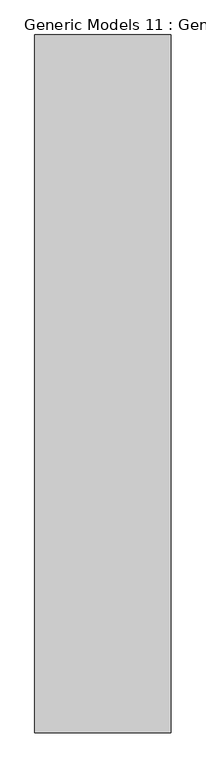
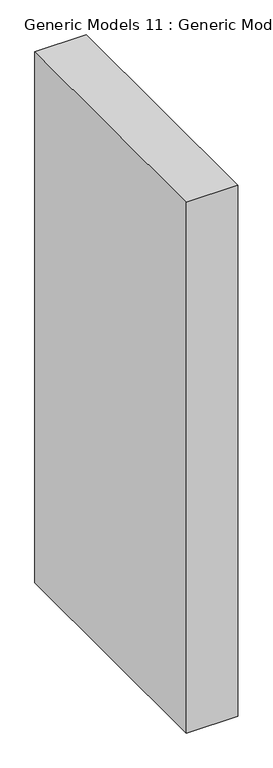
"""IFC4 building model written with IfcOpenShell, lengths in millimetres: proxy geometry, Generic Models 11 : Generic Models 11."""

from ifc_helpers import new_model, si_unit, frame, origin, place, context, project, spatial, polyline, outline, extrude, source, transform, mapped, element, save


def generic_models_11_generic_models_11_7edcfdbd(model_context):
    return source(origin(), model_context, "Body", "SweptSolid", [
        extrude(outline(polyline([(-10749.6371373, -2516.661407), (-10521.0371373, -2516.661407), (-10521.0371373, -3685.061407), (-10749.6371373, -3685.061407), (-10749.6371373, -2516.661407)])), frame((0.0, 0.0, 3657.6), z_axis=(0.0, 0.0, 1.0), x_axis=(1.0, 0.0, 0.0)), (0.0, 0.0, 1.0), 2498.1270621),
    ])


if __name__ == "__main__":
    model = new_model("IFC4")
    model_context = context("Model", 3, world=origin())
    ifc_project = project(units=[si_unit("LENGTHUNIT", "METRE", prefix="MILLI")], contexts=[model_context])
    site = spatial("IfcSite", under=ifc_project)
    building = spatial("IfcBuilding", under=site)
    placement = place(None, origin())
    generic_models_11_generic_models_11_shape = generic_models_11_generic_models_11_7edcfdbd(model_context)
    element("IfcBuildingElementProxy", 1, Name="Generic Models 11 : Generic Models 11", ObjectType="Generic Models 11 : Generic Models 11", at=placement, inside=building, context=model_context, shape_type="MappedRepresentation", body=[
        mapped(generic_models_11_generic_models_11_shape, transform((0.0, 0.0, 0.0), x_axis=(1.0, 0.0, 0.0), y_axis=(0.0, 1.0, 0.0), z_axis=(0.0, 0.0, 1.0))),
    ])
    save(model, "model.ifc")

# Revit data of these elements
# Element 1 (IfcBuildingElementProxy, "Generic Models 11 : Generic Models 11")
#   Materials on its faces: "Gypsum Wall Board"
# Materials
#   "Gypsum Wall Board": class "Generic", colour RGB 127 127 127, transparency 0, Description = "Gypsum Wall Board", Cost = 0
